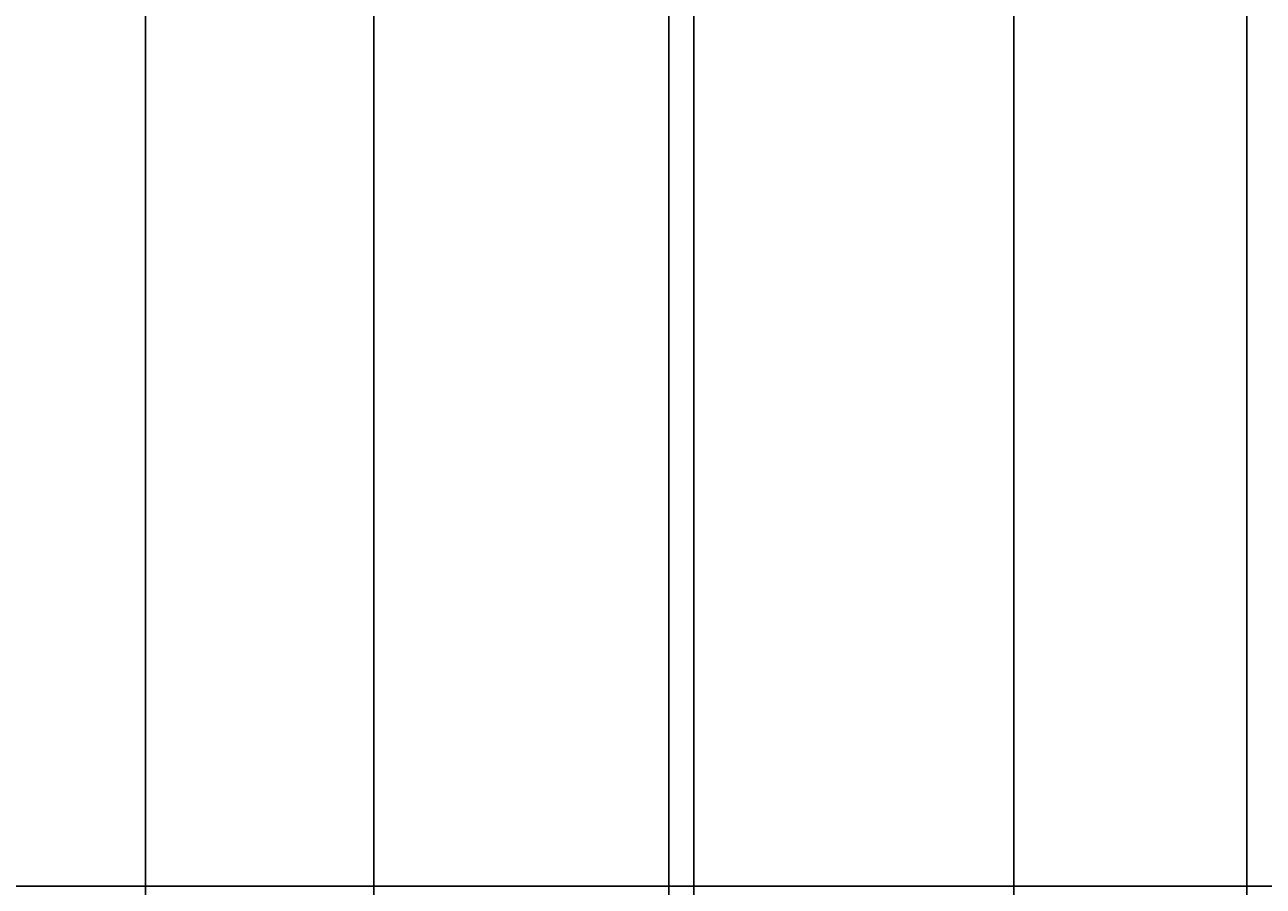
# Model space of a CAD drawing. Units: inches. Extents: x 2812 to 3051, y 1398 to 1659.
# Tile 14 of 65: x 2880 to 2911, y 1416 to 1437. Entities that reach past the tile are written whole.
import ezdxf

# ---------------------------------------------------------------- set-up
doc = ezdxf.new("R2010")
doc.units = ezdxf.units.IN
doc.layers.add('A-ANNO-DIMS', color=2, linetype='Continuous', lineweight=18)
doc.styles.get("Standard").update_dxf_attribs({"font": 'arial.ttf'})
doc.dimstyles.get("Standard").update_dxf_attribs({"dimtxt": 0.18, "dimasz": 0.18, "dimexe": 0.18, "dimexo": 0.0625, "dimgap": 0.09, "dimtad": 0, "dimtih": 1, "dimtoh": 1, "dimdec": 4, "dimzin": 0, "dimdsep": 46, "dimtxsty": 'Standard', "dimcen": 0.09, "dimadec": 0, "dimazin": 0, "dimtfac": 1, "dimtdec": 4, "dimtofl": 0, "dimtmove": 0, "dimatfit": 3, "dimfxl": 1, "dimtolj": 1, "dimtzin": 0, "dimarcsym": 0})

# ---------------------------------------------------------------- blocks, each defined once
blk = doc.blocks.new('*D29')
at = {"layer": 'A-ANNO-DIMS', "color": 0, "lineweight": -2, "transparency": 16777216}
for p, q in [((2910.742, 1598.757), (2910.742, 1397.505)), ((2883.385, 1559.757), (2883.385, 1397.505)), ((2883.565, 1397.685), (2896.598, 1397.685)), ((2910.562, 1397.685), (2897.528, 1397.685))]:
    blk.add_line(p, q, dxfattribs=at)
at = {"layer": 'A-ANNO-DIMS', "color": 0, "transparency": 16777216}
for points in [[(2883.565, 1397.715), (2883.565, 1397.655), (2883.385, 1397.685)], [(2910.562, 1397.715), (2910.562, 1397.655), (2910.742, 1397.685)]]:
    blk.add_solid(points, dxfattribs=at)
at = {"layer": 'Defpoints', "color": 0, "transparency": 16777216}
for p in [(2910.742, 1598.82), (2883.385, 1559.82), (2910.742, 1397.685)]:
    blk.add_point(p, dxfattribs=at)
at = {"layer": 'A-ANNO-DIMS', "color": 0, "transparency": 16777216, "insert": (2897.063, 1397.685), "char_height": 0.18, "attachment_point": 5}
blk.add_mtext('\\A1;27.357', dxfattribs=at)
blk = doc.blocks.new('*D44')
at = {"layer": 'A-ANNO-DIMS', "color": 0, "lineweight": -2, "transparency": 16777216}
for p, q in [((2850.748, 1487.973), (2850.748, 1397.505)), ((2896.385, 1487.973), (2896.385, 1397.505)), ((2850.928, 1397.685), (2873.17, 1397.685)), ((2896.205, 1397.685), (2873.964, 1397.685))]:
    blk.add_line(p, q, dxfattribs=at)
at = {"layer": 'A-ANNO-DIMS', "color": 0, "transparency": 16777216}
for points in [[(2850.928, 1397.715), (2850.928, 1397.655), (2850.748, 1397.685)], [(2896.205, 1397.715), (2896.205, 1397.655), (2896.385, 1397.685)]]:
    blk.add_solid(points, dxfattribs=at)
at = {"layer": 'Defpoints', "color": 0, "transparency": 16777216}
for p in [(2850.748, 1488.035), (2896.385, 1488.035), (2896.385, 1397.685)]:
    blk.add_point(p, dxfattribs=at)
at = {"layer": 'A-ANNO-DIMS', "color": 0, "transparency": 16777216, "insert": (2873.567, 1397.685), "char_height": 0.18, "attachment_point": 5}
blk.add_mtext('\\A1;45.64', dxfattribs=at)
blk = doc.blocks.new('*D45')
at = {"layer": 'A-ANNO-DIMS', "color": 0, "lineweight": -2, "transparency": 16777216}
for p, q in [((2896.385, 1487.973), (2896.385, 1397.505)), ((2941.385, 1487.973), (2941.385, 1397.505)), ((2896.565, 1397.685), (2918.662, 1397.685)), ((2941.205, 1397.685), (2919.108, 1397.685))]:
    blk.add_line(p, q, dxfattribs=at)
at = {"layer": 'A-ANNO-DIMS', "color": 0, "transparency": 16777216}
for points in [[(2896.565, 1397.715), (2896.565, 1397.655), (2896.385, 1397.685)], [(2941.205, 1397.715), (2941.205, 1397.655), (2941.385, 1397.685)]]:
    blk.add_solid(points, dxfattribs=at)
at = {"layer": 'Defpoints', "color": 0, "transparency": 16777216}
for p in [(2896.385, 1488.035), (2941.385, 1488.035), (2941.385, 1397.685)]:
    blk.add_point(p, dxfattribs=at)
at = {"layer": 'A-ANNO-DIMS', "color": 0, "transparency": 16777216, "insert": (2918.885, 1397.685), "char_height": 0.18, "attachment_point": 5}
blk.add_mtext('\\A1;45', dxfattribs=at)
blk = doc.blocks.new('*D56')
at = {"layer": 'A-ANNO-DIMS', "color": 0, "lineweight": -2, "transparency": 16777216}
for p, q in [((2880.322, 1452.035), (2811.806, 1452.035)), ((2811.986, 1451.855), (2811.986, 1434.217)), ((2811.986, 1416.215), (2811.986, 1433.853)), ((2952.322, 1416.035), (2811.806, 1416.035))]:
    blk.add_line(p, q, dxfattribs=at)
at = {"layer": 'A-ANNO-DIMS', "color": 0, "transparency": 16777216}
for points in [[(2811.956, 1451.855), (2812.016, 1451.855), (2811.986, 1452.035)], [(2811.956, 1416.215), (2812.016, 1416.215), (2811.986, 1416.035)]]:
    blk.add_solid(points, dxfattribs=at)
at = {"layer": 'Defpoints', "color": 0, "transparency": 16777216}
for p in [(2811.986, 1452.035), (2880.385, 1452.035), (2952.385, 1416.035)]:
    blk.add_point(p, dxfattribs=at)
at = {"layer": 'A-ANNO-DIMS', "color": 0, "transparency": 16777216, "insert": (2811.986, 1434.035), "char_height": 0.18, "attachment_point": 5}
blk.add_mtext('\\A1;36', dxfattribs=at)
blk = doc.blocks.new('*D60')
at = {"layer": 'A-ANNO-DIMS', "color": 0, "lineweight": -2, "transparency": 16777216}
for p, q in [((2889.058, 1466.34), (2889.058, 1397.505)), ((2897.002, 1457.364), (2897.002, 1397.505)), ((2889.238, 1397.685), (2892.637, 1397.685)), ((2896.822, 1397.685), (2893.422, 1397.685))]:
    blk.add_line(p, q, dxfattribs=at)
at = {"layer": 'A-ANNO-DIMS', "color": 0, "transparency": 16777216}
for points in [[(2889.238, 1397.715), (2889.238, 1397.655), (2889.058, 1397.685)], [(2896.822, 1397.715), (2896.822, 1397.655), (2897.002, 1397.685)]]:
    blk.add_solid(points, dxfattribs=at)
at = {"layer": 'Defpoints', "color": 0, "transparency": 16777216}
for p in [(2889.058, 1466.402), (2897.002, 1457.426), (2897.002, 1397.685)]:
    blk.add_point(p, dxfattribs=at)
at = {"layer": 'A-ANNO-DIMS', "color": 0, "transparency": 16777216, "insert": (2893.03, 1397.685), "char_height": 0.18, "attachment_point": 5}
blk.add_mtext('\\A1;7.944', dxfattribs=at)
blk = doc.blocks.new('*D61')
at = {"layer": 'A-ANNO-DIMS', "color": 0, "lineweight": -2, "transparency": 16777216}
for p, q in [((2897.002, 1457.364), (2897.002, 1397.505)), ((2904.955, 1447.364), (2904.955, 1397.505)), ((2897.182, 1397.685), (2900.586, 1397.685)), ((2904.775, 1397.685), (2901.372, 1397.685))]:
    blk.add_line(p, q, dxfattribs=at)
at = {"layer": 'A-ANNO-DIMS', "color": 0, "transparency": 16777216}
for points in [[(2897.182, 1397.715), (2897.182, 1397.655), (2897.002, 1397.685)], [(2904.775, 1397.715), (2904.775, 1397.655), (2904.955, 1397.685)]]:
    blk.add_solid(points, dxfattribs=at)
at = {"layer": 'Defpoints', "color": 0, "transparency": 16777216}
for p in [(2897.002, 1457.426), (2904.955, 1447.426), (2904.955, 1397.685)]:
    blk.add_point(p, dxfattribs=at)
at = {"layer": 'A-ANNO-DIMS', "color": 0, "transparency": 16777216, "insert": (2900.979, 1397.685), "char_height": 0.18, "attachment_point": 5}
blk.add_mtext('\\A1;7.953', dxfattribs=at)
blk = doc.blocks.new('*D62')
at = {"layer": 'A-ANNO-DIMS', "color": 0, "lineweight": -2, "transparency": 16777216}
for p, q in [((2904.955, 1447.364), (2904.955, 1397.505)), ((2911.558, 1437.364), (2911.558, 1397.505)), ((2905.135, 1397.685), (2907.862, 1397.685)), ((2911.378, 1397.685), (2908.651, 1397.685))]:
    blk.add_line(p, q, dxfattribs=at)
at = {"layer": 'A-ANNO-DIMS', "color": 0, "transparency": 16777216}
for points in [[(2905.135, 1397.715), (2905.135, 1397.655), (2904.955, 1397.685)], [(2911.378, 1397.715), (2911.378, 1397.655), (2911.558, 1397.685)]]:
    blk.add_solid(points, dxfattribs=at)
at = {"layer": 'Defpoints', "color": 0, "transparency": 16777216}
for p in [(2904.955, 1447.426), (2911.558, 1437.426), (2911.558, 1397.685)]:
    blk.add_point(p, dxfattribs=at)
at = {"layer": 'A-ANNO-DIMS', "color": 0, "transparency": 16777216, "insert": (2908.256, 1397.685), "char_height": 0.18, "attachment_point": 5}
blk.add_mtext('\\A1;6.603', dxfattribs=at)
blk = doc.blocks.new('*D75')
at = {"layer": 'A-ANNO-DIMS', "color": 0, "lineweight": -2, "transparency": 16777216}
for p, q in [((2963.812, 1448.474), (2811.806, 1448.474)), ((2811.986, 1448.294), (2811.986, 1432.437)), ((2811.986, 1416.215), (2811.986, 1432.073)), ((2961.322, 1416.035), (2811.806, 1416.035))]:
    blk.add_line(p, q, dxfattribs=at)
at = {"layer": 'A-ANNO-DIMS', "color": 0, "transparency": 16777216}
for points in [[(2811.956, 1448.294), (2812.016, 1448.294), (2811.986, 1448.474)], [(2811.956, 1416.215), (2812.016, 1416.215), (2811.986, 1416.035)]]:
    blk.add_solid(points, dxfattribs=at)
at = {"layer": 'Defpoints', "color": 0, "transparency": 16777216}
for p in [(2811.986, 1448.474), (2963.874, 1448.474), (2961.385, 1416.035)]:
    blk.add_point(p, dxfattribs=at)
at = {"layer": 'A-ANNO-DIMS', "color": 0, "transparency": 16777216, "insert": (2811.986, 1432.255), "char_height": 0.18, "attachment_point": 5}
blk.add_mtext('\\A1;32.44', dxfattribs=at)

msp = doc.modelspace()

# ---------------------------------------------------------------- dimensions: what is measured, and where the dimension line sits
at = {"layer": 'A-ANNO-DIMS'}
for base, p1, p2, override, picture, middle in [((2910.7415, 1397.6854), (2883.3849, 1559.82), (2910.7415, 1598.82), {"dimdec": 3, "dimlfac": 1, "dimrnd": 0, "dimzin": 0, "dimdsep": 46, "dimlunit": 2}, '*D29', (2897.0632, 1397.6854)), ((2896.3849, 1397.6854), (2850.7485, 1488.0354), (2896.3849, 1488.0354), {"dimdec": 2, "dimlfac": 1, "dimrnd": 0, "dimzin": 0, "dimdsep": 46, "dimlunit": 2}, '*D44', (2873.5667, 1397.6854)), ((2941.3849, 1397.6854), (2896.3849, 1488.0354), (2941.3849, 1488.0354), {"dimdec": 0, "dimlfac": 1, "dimrnd": 0, "dimzin": 0, "dimdsep": 46, "dimlunit": 2}, '*D45', (2918.8849, 1397.6854)), ((2897.0021, 1397.6854), (2889.0577, 1466.4024), (2897.0021, 1457.4265), {"dimdec": 3, "dimlfac": 1, "dimrnd": 0, "dimzin": 0, "dimdsep": 46, "dimlunit": 2}, '*D60', (2893.0299, 1397.6854)), ((2904.9551, 1397.6854), (2897.0021, 1457.4265), (2904.9551, 1447.4265), {"dimdec": 3, "dimlfac": 1, "dimrnd": 0, "dimzin": 0, "dimdsep": 46, "dimlunit": 2}, '*D61', (2900.9786, 1397.6854)), ((2911.5577, 1397.6854), (2904.9551, 1447.4265), (2911.5577, 1437.4265), {"dimdec": 3, "dimlfac": 1, "dimrnd": 0, "dimzin": 0, "dimdsep": 46, "dimlunit": 2}, '*D62', (2908.2564, 1397.6854))]:
    dim = msp.add_linear_dim(base=base, p1=p1, p2=p2, dimstyle='Standard', override=override, dxfattribs=at)
    dim.commit()
    dim.dimension.update_dxf_attribs({"geometry": picture, "text_midpoint": middle})
for base, p1, p2, override, picture, middle in [((2811.9855, 1452.0354), (2952.3849, 1416.0354), (2880.3849, 1452.0354), {"dimdec": 0, "dimlfac": 1, "dimrnd": 0, "dimzin": 0, "dimdsep": 46, "dimlunit": 2}, '*D56', (2811.9855, 1434.0354)), ((2811.9855, 1448.4738), (2961.3849, 1416.0354), (2963.8741, 1448.4738), {"dimdec": 2, "dimlfac": 1, "dimrnd": 0, "dimzin": 0, "dimdsep": 46, "dimlunit": 2}, '*D75', (2811.9855, 1432.2546))]:
    dim = msp.add_linear_dim(base=base, p1=p1, p2=p2, angle=90, dimstyle='Standard', override=override, dxfattribs=at)
    dim.commit()
    dim.dimension.update_dxf_attribs({"geometry": picture, "text_midpoint": middle})

doc.saveas('drawing.dxf')
